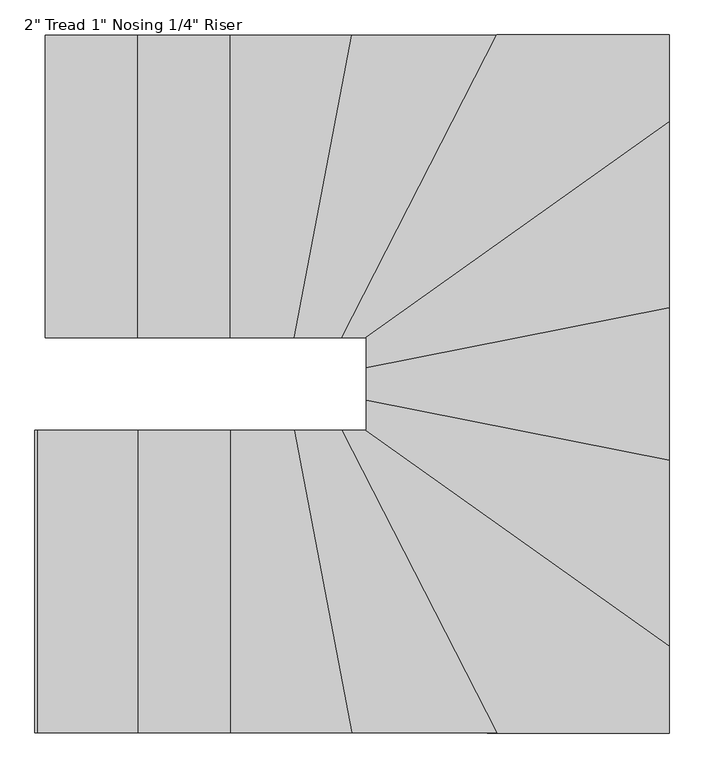
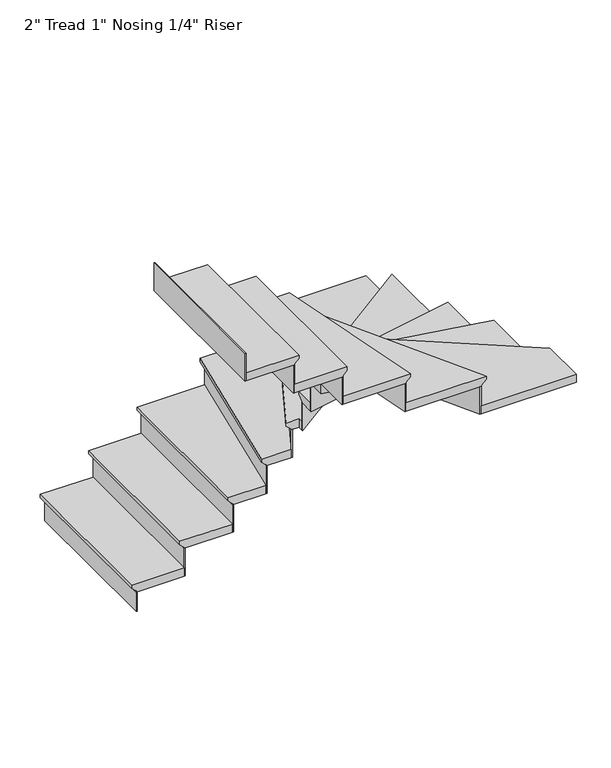
"""IFC4 building model written with IfcOpenShell, lengths in millimetres: stair flight geometry."""

from ifc_helpers import new_model, si_unit, origin, place, context, project, spatial, faceted_brep, source, transform, mapped, element, save


def stair_flight_89efee2b(model_context):
    return source(origin(), model_context, "Body", "Brep", [
        faceted_brep([(-11800.6429074, -1535.9895999, 488.95), (-11800.6429074, -1535.9895999, 508.0), (-11800.6429074, -621.5895999, 508.0), (-11800.6429074, -621.5895999, 488.95), (-11775.2429074, -1535.9895999, 463.55), (-11775.2429074, -621.5895999, 463.55), (-11495.8429074, -1535.9895999, 508.0), (-11495.8429074, -621.5895999, 508.0), (-11775.2429074, -621.5895999, 457.2), (-11495.8429074, -621.5895999, 457.2), (-11495.8429074, -1535.9895999, 457.2), (-11775.2429074, -1535.9895999, 457.2)], [[[0, 1, 2, 3]], [[4, 0, 3, 5]], [[2, 1, 6, 7]], [[8, 9, 10, 11]], [[2, 7, 9, 8, 5, 3]], [[8, 11, 4, 5]], [[6, 1, 0, 4, 11, 10]], [[7, 6, 10, 9]]]),
        faceted_brep([(-11775.2429074, -1535.9895999, 457.2), (-11775.2429074, -1535.9895999, 338.6666667), (-11768.8929074, -1535.9895999, 338.6666667), (-11768.8929074, -1535.9895999, 457.2), (-11775.2429074, -621.5895999, 457.2), (-11768.8929074, -621.5895999, 457.2), (-11768.8929074, -621.5895999, 338.6666667), (-11775.2429074, -621.5895999, 338.6666667)], [[[0, 1, 2, 3]], [[4, 5, 6, 7]], [[1, 0, 4, 7]], [[2, 1, 7, 6]], [[3, 2, 6, 5]], [[0, 3, 5, 4]]]),
        faceted_brep([(-11495.8429074, -1535.9895999, 626.5333333), (-11495.8429074, -1535.9895999, 457.2), (-11489.4929074, -1535.9895999, 457.2), (-11489.4929074, -1535.9895999, 626.5333333), (-11495.8429074, -621.5895999, 626.5333333), (-11489.4929074, -621.5895999, 626.5333333), (-11489.4929074, -621.5895999, 457.2), (-11495.8429074, -621.5895999, 457.2)], [[[0, 1, 2, 3]], [[4, 5, 6, 7]], [[1, 0, 4, 7]], [[2, 1, 7, 6]], [[3, 2, 6, 5]], [[0, 3, 5, 4]]]),
        faceted_brep([(-11521.2429074, -621.5895999, 677.3333333), (-11521.2429074, -1535.9895999, 677.3333333), (-11216.4429074, -1535.9895999, 677.3333333), (-11216.4429074, -621.5895999, 677.3333333), (-11495.8429074, -621.5895999, 626.5333333), (-11216.4429074, -621.5895999, 626.5333333), (-11216.4429074, -1535.9895999, 626.5333333), (-11495.8429074, -1535.9895999, 626.5333333), (-11495.8429074, -621.5895999, 632.8833333), (-11521.2429074, -621.5895999, 658.2833333), (-11495.8429074, -1535.9895999, 632.8833333), (-11521.2429074, -1535.9895999, 658.2833333)], [[[0, 1, 2, 3]], [[4, 5, 6, 7]], [[0, 3, 5, 4, 8, 9]], [[4, 7, 10, 8]], [[2, 1, 11, 10, 7, 6]], [[3, 2, 6, 5]], [[11, 1, 0, 9]], [[10, 11, 9, 8]]]),
        faceted_brep([(-11216.4429074, -1535.9895999, 795.8666667), (-11216.4429074, -1535.9895999, 626.5333333), (-11210.0929074, -1535.9895999, 626.5333333), (-11210.0929074, -1535.9895999, 795.8666667), (-11216.4429074, -621.5895999, 795.8666667), (-11210.0929074, -621.5895999, 795.8666667), (-11210.0929074, -621.5895999, 626.5333333), (-11216.4429074, -621.5895999, 626.5333333)], [[[0, 1, 2, 3]], [[4, 5, 6, 7]], [[1, 0, 4, 7]], [[2, 1, 7, 6]], [[3, 2, 6, 5]], [[0, 3, 5, 4]]]),
        faceted_brep([(-11241.8429074, -621.5895999, 846.6666667), (-11241.8429074, -1535.9895999, 846.6666667), (-11023.0627678, -1535.9895999, 846.6666667), (-10850.1224695, -621.5895999, 846.6666667), (-11216.4429074, -621.5895999, 795.8666667), (-10850.1224695, -621.5895999, 795.8666667), (-11023.0627678, -1535.9895999, 795.8666667), (-11216.4429074, -1535.9895999, 795.8666667), (-11216.4429074, -621.5895999, 802.2166667), (-11241.8429074, -621.5895999, 827.6166667), (-11216.4429074, -1535.9895999, 802.2166667), (-11241.8429074, -1535.9895999, 827.6166667)], [[[0, 1, 2, 3]], [[4, 5, 6, 7]], [[0, 3, 5, 4, 8, 9]], [[4, 7, 10, 8]], [[2, 1, 11, 10, 7, 6]], [[3, 2, 6, 5]], [[11, 1, 0, 9]], [[10, 11, 9, 8]]]),
        faceted_brep([(-11023.0627678, -1535.9895999, 965.2), (-11023.0627678, -1535.9895999, 795.8666667), (-11016.6001956, -1535.9895999, 795.8666667), (-11016.6001956, -1535.9895999, 965.2), (-10850.1224695, -621.5895999, 965.2), (-10843.6598973, -621.5895999, 965.2), (-10843.6598973, -621.5895999, 795.8666667), (-10850.1224695, -621.5895999, 795.8666667)], [[[0, 1, 2, 3]], [[4, 5, 6, 7]], [[1, 0, 4, 7]], [[2, 1, 7, 6]], [[3, 2, 6, 5]], [[0, 3, 5, 4]]]),
        faceted_brep([(-10875.9727582, -621.5895999, 1016.0), (-11048.9130565, -1535.9895999, 1016.0), (-10877.4351875, -1535.9895999, 1016.0), (-10408.6105662, -621.5895999, 1016.0), (-10850.1224695, -621.5895999, 965.2), (-10408.6105662, -621.5895999, 965.2), (-10877.4351875, -1535.9895999, 965.2), (-11023.0627678, -1535.9895999, 965.2), (-10850.1224695, -621.5895999, 971.55), (-10875.9727582, -621.5895999, 996.95), (-11023.0627678, -1535.9895999, 971.55), (-11048.9130565, -1535.9895999, 996.95)], [[[0, 1, 2, 3]], [[4, 5, 6, 7]], [[0, 3, 5, 4, 8, 9]], [[4, 7, 10, 8]], [[2, 1, 11, 10, 7, 6]], [[3, 2, 6, 5]], [[11, 1, 0, 9]], [[10, 11, 9, 8]]]),
        faceted_brep([(-10877.4351875, -1535.9895999, 1134.5333333), (-10877.4351875, -1535.9895999, 965.2), (-10870.2992044, -1535.9895999, 965.2), (-10870.2992044, -1535.9895999, 1134.5333333), (-10408.6105662, -621.5895999, 1134.5333333), (-10401.4745831, -621.5895999, 1134.5333333), (-10401.4745831, -621.5895999, 965.2), (-10408.6105662, -621.5895999, 965.2)], [[[0, 1, 2, 3]], [[4, 5, 6, 7]], [[1, 0, 4, 7]], [[2, 1, 7, 6]], [[3, 2, 6, 5]], [[0, 3, 5, 4]]]),
        faceted_brep([(-9917.3112155, -915.2707336, 1185.3333333), (-9917.3112155, -621.5895999, 1185.3333333), (-10437.1544987, -621.5895999, 1185.3333333), (-10905.9791201, -1535.9895999, 1185.3333333), (-10831.7112155, -1535.9895999, 1185.3333333), (-10831.7112155, -1565.5446827, 1185.3333333), (-9917.3112155, -621.5895999, 1134.5333333), (-9917.3112155, -915.2707336, 1134.5333333), (-10831.7112155, -1565.5446827, 1134.5333333), (-10831.7112155, -1535.9895999, 1134.5333333), (-10877.4351875, -1535.9895999, 1134.5333333), (-10408.6105662, -621.5895999, 1134.5333333), (-10877.4351875, -1535.9895999, 1140.8833333), (-10408.6105662, -621.5895999, 1140.8833333), (-10905.9791201, -1535.9895999, 1166.2833333), (-10437.1544987, -621.5895999, 1166.2833333)], [[[0, 1, 2, 3, 4, 5]], [[6, 7, 8, 9, 10, 11]], [[1, 0, 7, 6]], [[11, 10, 12, 13]], [[4, 3, 14, 12, 10, 9]], [[0, 5, 8, 7]], [[14, 3, 2, 15]], [[12, 14, 15, 13]], [[2, 1, 6, 11, 13, 15]], [[5, 4, 9, 8]]]),
        faceted_brep([(-10831.7112155, -1565.5446827, 1303.8666667), (-10831.7112155, -1565.5446827, 1134.5333333), (-10831.7112155, -1573.3366575, 1134.5333333), (-10831.7112155, -1573.3366575, 1303.8666667), (-9917.3112155, -915.2707336, 1303.8666667), (-9917.3112155, -923.0627084, 1303.8666667), (-9917.3112155, -923.0627084, 1134.5333333), (-9917.3112155, -915.2707336, 1134.5333333)], [[[0, 1, 2, 3]], [[4, 5, 6, 7]], [[1, 0, 4, 7]], [[2, 1, 7, 6]], [[3, 2, 6, 5]], [[0, 3, 5, 4]]]),
        faceted_brep([(-9917.3112155, -884.1028344, 1354.6666667), (-10831.7112155, -1534.3767836, 1354.6666667), (-10831.7112155, -1651.9987698, 1354.6666667), (-9917.3112155, -1471.7579135, 1354.6666667), (-9917.3112155, -915.2707336, 1303.8666667), (-9917.3112155, -1471.7579135, 1303.8666667), (-10831.7112155, -1651.9987698, 1303.8666667), (-10831.7112155, -1565.5446827, 1303.8666667), (-9917.3112155, -915.2707336, 1310.2166667), (-9917.3112155, -884.1028344, 1335.6166667), (-10831.7112155, -1565.5446827, 1310.2166667), (-10831.7112155, -1534.3767836, 1335.6166667)], [[[0, 1, 2, 3]], [[4, 5, 6, 7]], [[0, 3, 5, 4, 8, 9]], [[4, 7, 10, 8]], [[3, 2, 6, 5]], [[11, 1, 0, 9]], [[10, 11, 9, 8]], [[2, 1, 11, 10, 7, 6]]]),
        faceted_brep([(-10831.7112155, -1651.9987698, 1473.2), (-10831.7112155, -1651.9987698, 1303.8666667), (-10831.7112155, -1658.4709552, 1303.8666667), (-10831.7112155, -1658.4709552, 1473.2), (-9917.3112155, -1471.7579135, 1473.2), (-9917.3112155, -1478.2300989, 1473.2), (-9917.3112155, -1478.2300989, 1303.8666667), (-9917.3112155, -1471.7579135, 1303.8666667)], [[[0, 1, 2, 3]], [[4, 5, 6, 7]], [[1, 0, 4, 7]], [[2, 1, 7, 6]], [[3, 2, 6, 5]], [[0, 3, 5, 4]]]),
        faceted_brep([(-9917.3112155, -1445.8691717, 1524.0), (-10831.7112155, -1626.1100281, 1524.0), (-10831.7112155, -1751.1579135, 1524.0), (-9917.3112155, -1931.3987698, 1524.0), (-9917.3112155, -1471.7579135, 1473.2), (-9917.3112155, -1931.3987698, 1473.2), (-10831.7112155, -1751.1579135, 1473.2), (-10831.7112155, -1651.9987698, 1473.2), (-9917.3112155, -1471.7579135, 1479.55), (-9917.3112155, -1445.8691717, 1504.95), (-10831.7112155, -1651.9987698, 1479.55), (-10831.7112155, -1626.1100281, 1504.95)], [[[0, 1, 2, 3]], [[4, 5, 6, 7]], [[0, 3, 5, 4, 8, 9]], [[4, 7, 10, 8]], [[2, 1, 11, 10, 7, 6]], [[3, 2, 6, 5]], [[11, 1, 0, 9]], [[10, 11, 9, 8]]]),
        faceted_brep([(-10831.7112155, -1751.1579135, 1642.5333333), (-10831.7112155, -1751.1579135, 1473.2), (-10831.7112155, -1757.6300989, 1473.2), (-10831.7112155, -1757.6300989, 1642.5333333), (-9917.3112155, -1931.3987698, 1642.5333333), (-9917.3112155, -1937.8709552, 1642.5333333), (-9917.3112155, -1937.8709552, 1473.2), (-9917.3112155, -1931.3987698, 1473.2)], [[[0, 1, 2, 3]], [[4, 5, 6, 7]], [[1, 0, 4, 7]], [[2, 1, 7, 6]], [[3, 2, 6, 5]], [[0, 3, 5, 4]]]),
        faceted_brep([(-9917.3112155, -1905.5100281, 1693.3333333), (-10831.7112155, -1725.2691717, 1693.3333333), (-10831.7112155, -1815.3895999, 1693.3333333), (-10877.80669, -1815.3895999, 1693.3333333), (-9917.3112155, -2498.4442646, 1693.3333333), (-9917.3112155, -1931.3987698, 1642.5333333), (-9917.3112155, -2498.4442646, 1642.5333333), (-10877.80669, -1815.3895999, 1642.5333333), (-10831.7112155, -1815.3895999, 1642.5333333), (-10831.7112155, -1751.1579135, 1642.5333333), (-9917.3112155, -1931.3987698, 1648.8833333), (-9917.3112155, -1905.5100281, 1674.2833333), (-10831.7112155, -1751.1579135, 1648.8833333), (-10831.7112155, -1725.2691717, 1674.2833333)], [[[0, 1, 2, 3, 4]], [[5, 6, 7, 8, 9]], [[0, 4, 6, 5, 10, 11]], [[5, 9, 12, 10]], [[3, 2, 8, 7]], [[4, 3, 7, 6]], [[13, 1, 0, 11]], [[12, 13, 11, 10]], [[2, 1, 13, 12, 9, 8]]]),
        faceted_brep([(-10877.80669, -1815.3895999, 1811.8666667), (-10877.80669, -1815.3895999, 1642.5333333), (-10888.7635825, -1815.3895999, 1642.5333333), (-10888.7635825, -1815.3895999, 1811.8666667), (-9917.3112155, -2498.4442646, 1811.8666667), (-9917.3112155, -2506.2362394, 1811.8666667), (-9917.3112155, -2506.2362394, 1642.5333333), (-9917.3112155, -2498.4442646, 1642.5333333)], [[[0, 1, 2, 3]], [[4, 5, 6, 7]], [[1, 0, 4, 7]], [[2, 1, 7, 6]], [[3, 2, 6, 5]], [[0, 3, 5, 4]]]),
        faceted_brep([(-10465.6984313, -2729.7895999, 1862.6666667), (-9917.3112155, -2729.7895999, 1862.6666667), (-9917.3112155, -2467.2763654, 1862.6666667), (-10833.9791201, -1815.3895999, 1862.6666667), (-10934.5230526, -1815.3895999, 1862.6666667), (-9917.3112155, -2729.7895999, 1811.8666667), (-10465.6984313, -2729.7895999, 1811.8666667), (-10934.5230526, -1815.3895999, 1811.8666667), (-10877.80669, -1815.3895999, 1811.8666667), (-9917.3112155, -2498.4442646, 1811.8666667), (-10877.80669, -1815.3895999, 1818.2166667), (-9917.3112155, -2498.4442646, 1818.2166667), (-10833.9791201, -1815.3895999, 1843.6166667), (-9917.3112155, -2467.2763654, 1843.6166667)], [[[0, 1, 2, 3, 4]], [[5, 6, 7, 8, 9]], [[1, 0, 6, 5]], [[9, 8, 10, 11]], [[4, 3, 12, 10, 8, 7]], [[0, 4, 7, 6]], [[12, 3, 2, 13]], [[10, 12, 13, 11]], [[2, 1, 5, 9, 11, 13]]]),
        faceted_brep([(-10934.5230526, -1815.3895999, 1981.2), (-10934.5230526, -1815.3895999, 1811.8666667), (-10941.6590357, -1815.3895999, 1811.8666667), (-10941.6590357, -1815.3895999, 1981.2), (-10465.6984313, -2729.7895999, 1981.2), (-10472.8344144, -2729.7895999, 1981.2), (-10472.8344144, -2729.7895999, 1811.8666667), (-10465.6984313, -2729.7895999, 1811.8666667)], [[[0, 1, 2, 3]], [[4, 5, 6, 7]], [[1, 0, 4, 7]], [[2, 1, 7, 6]], [[3, 2, 6, 5]], [[0, 3, 5, 4]]]),
        faceted_brep([(-10437.1544987, -2729.7895999, 2032.0), (-10905.9791201, -1815.3895999, 2032.0), (-11074.7633453, -1815.3895999, 2032.0), (-10901.823047, -2729.7895999, 2032.0), (-10465.6984313, -2729.7895999, 1981.2), (-10901.823047, -2729.7895999, 1981.2), (-11074.7633453, -1815.3895999, 1981.2), (-10934.5230526, -1815.3895999, 1981.2), (-10465.6984313, -2729.7895999, 1987.55), (-10437.1544987, -2729.7895999, 2012.95), (-10934.5230526, -1815.3895999, 1987.55), (-10905.9791201, -1815.3895999, 2012.95)], [[[0, 1, 2, 3]], [[4, 5, 6, 7]], [[0, 3, 5, 4, 8, 9]], [[4, 7, 10, 8]], [[2, 1, 11, 10, 7, 6]], [[3, 2, 6, 5]], [[11, 1, 0, 9]], [[10, 11, 9, 8]]]),
        faceted_brep([(-11074.7633453, -1815.3895999, 2150.5333333), (-11074.7633453, -1815.3895999, 1981.2), (-11081.2259175, -1815.3895999, 1981.2), (-11081.2259175, -1815.3895999, 2150.5333333), (-10901.823047, -2729.7895999, 2150.5333333), (-10908.2856191, -2729.7895999, 2150.5333333), (-10908.2856191, -2729.7895999, 1981.2), (-10901.823047, -2729.7895999, 1981.2)], [[[0, 1, 2, 3]], [[4, 5, 6, 7]], [[1, 0, 4, 7]], [[2, 1, 7, 6]], [[3, 2, 6, 5]], [[0, 3, 5, 4]]]),
        faceted_brep([(-10875.9727582, -2729.7895999, 2201.3333333), (-11048.9130565, -1815.3895999, 2201.3333333), (-11267.2429074, -1815.3895999, 2201.3333333), (-11267.2429074, -2729.7895999, 2201.3333333), (-10901.823047, -2729.7895999, 2150.5333333), (-11267.2429074, -2729.7895999, 2150.5333333), (-11267.2429074, -1815.3895999, 2150.5333333), (-11074.7633453, -1815.3895999, 2150.5333333), (-10901.823047, -2729.7895999, 2156.8833333), (-10875.9727582, -2729.7895999, 2182.2833333), (-11074.7633453, -1815.3895999, 2156.8833333), (-11048.9130565, -1815.3895999, 2182.2833333)], [[[0, 1, 2, 3]], [[4, 5, 6, 7]], [[0, 3, 5, 4, 8, 9]], [[4, 7, 10, 8]], [[2, 1, 11, 10, 7, 6]], [[3, 2, 6, 5]], [[11, 1, 0, 9]], [[10, 11, 9, 8]]]),
        faceted_brep([(-11267.2429074, -1815.3895999, 2319.8666667), (-11267.2429074, -1815.3895999, 2150.5333333), (-11273.5929074, -1815.3895999, 2150.5333333), (-11273.5929074, -1815.3895999, 2319.8666667), (-11267.2429074, -2729.7895999, 2319.8666667), (-11273.5929074, -2729.7895999, 2319.8666667), (-11273.5929074, -2729.7895999, 2150.5333333), (-11267.2429074, -2729.7895999, 2150.5333333)], [[[0, 1, 2, 3]], [[4, 5, 6, 7]], [[1, 0, 4, 7]], [[2, 1, 7, 6]], [[3, 2, 6, 5]], [[0, 3, 5, 4]]]),
        faceted_brep([(-11241.8429074, -2729.7895999, 2370.6666667), (-11241.8429074, -1815.3895999, 2370.6666667), (-11546.6429074, -1815.3895999, 2370.6666667), (-11546.6429074, -2729.7895999, 2370.6666667), (-11267.2429074, -2729.7895999, 2319.8666667), (-11546.6429074, -2729.7895999, 2319.8666667), (-11546.6429074, -1815.3895999, 2319.8666667), (-11267.2429074, -1815.3895999, 2319.8666667), (-11267.2429074, -2729.7895999, 2326.2166667), (-11241.8429074, -2729.7895999, 2351.6166667), (-11267.2429074, -1815.3895999, 2326.2166667), (-11241.8429074, -1815.3895999, 2351.6166667)], [[[0, 1, 2, 3]], [[4, 5, 6, 7]], [[0, 3, 5, 4, 8, 9]], [[4, 7, 10, 8]], [[2, 1, 11, 10, 7, 6]], [[3, 2, 6, 5]], [[11, 1, 0, 9]], [[10, 11, 9, 8]]]),
        faceted_brep([(-11546.6429074, -1815.3895999, 2489.2), (-11546.6429074, -1815.3895999, 2319.8666667), (-11552.9929074, -1815.3895999, 2319.8666667), (-11552.9929074, -1815.3895999, 2489.2), (-11546.6429074, -2729.7895999, 2489.2), (-11552.9929074, -2729.7895999, 2489.2), (-11552.9929074, -2729.7895999, 2319.8666667), (-11546.6429074, -2729.7895999, 2319.8666667)], [[[0, 1, 2, 3]], [[4, 5, 6, 7]], [[1, 0, 4, 7]], [[2, 1, 7, 6]], [[3, 2, 6, 5]], [[0, 3, 5, 4]]]),
        faceted_brep([(-11826.0429074, -1815.3895999, 2658.5333333), (-11826.0429074, -1815.3895999, 2489.2), (-11832.3929074, -1815.3895999, 2489.2), (-11832.3929074, -1815.3895999, 2658.5333333), (-11826.0429074, -2729.7895999, 2658.5333333), (-11832.3929074, -2729.7895999, 2658.5333333), (-11832.3929074, -2729.7895999, 2489.2), (-11826.0429074, -2729.7895999, 2489.2)], [[[0, 1, 2, 3]], [[4, 5, 6, 7]], [[1, 0, 4, 7]], [[2, 1, 7, 6]], [[3, 2, 6, 5]], [[0, 3, 5, 4]]]),
        faceted_brep([(-11521.2429074, -2729.7895999, 2540.0), (-11521.2429074, -1815.3895999, 2540.0), (-11826.0429074, -1815.3895999, 2540.0), (-11826.0429074, -2729.7895999, 2540.0), (-11546.6429074, -2729.7895999, 2489.2), (-11826.0429074, -2729.7895999, 2489.2), (-11826.0429074, -1815.3895999, 2489.2), (-11546.6429074, -1815.3895999, 2489.2), (-11546.6429074, -2729.7895999, 2495.55), (-11521.2429074, -2729.7895999, 2520.95), (-11546.6429074, -1815.3895999, 2495.55), (-11521.2429074, -1815.3895999, 2520.95)], [[[0, 1, 2, 3]], [[4, 5, 6, 7]], [[0, 3, 5, 4, 8, 9]], [[4, 7, 10, 8]], [[2, 1, 11, 10, 7, 6]], [[3, 2, 6, 5]], [[11, 1, 0, 9]], [[10, 11, 9, 8]]]),
    ])


if __name__ == "__main__":
    model = new_model("IFC4")
    model_context = context("Model", 3, world=origin())
    ifc_project = project(units=[si_unit("LENGTHUNIT", "METRE", prefix="MILLI")], contexts=[model_context])
    site = spatial("IfcSite", under=ifc_project)
    building = spatial("IfcBuilding", under=site)
    placement = place(None, origin())
    stair_flight_shape = stair_flight_89efee2b(model_context)
    element("IfcStairFlight", 1, ObjectType="2\" Tread 1\" Nosing 1/4\" Riser", at=placement, inside=building, context=model_context, shape_type="MappedRepresentation", body=[
        mapped(stair_flight_shape, transform((0.0, 0.0, 0.0), x_axis=(1.0, 0.0, 0.0), y_axis=(0.0, 1.0, 0.0), z_axis=(0.0, 0.0, 1.0))),
    ])
    save(model, "model.ifc")
